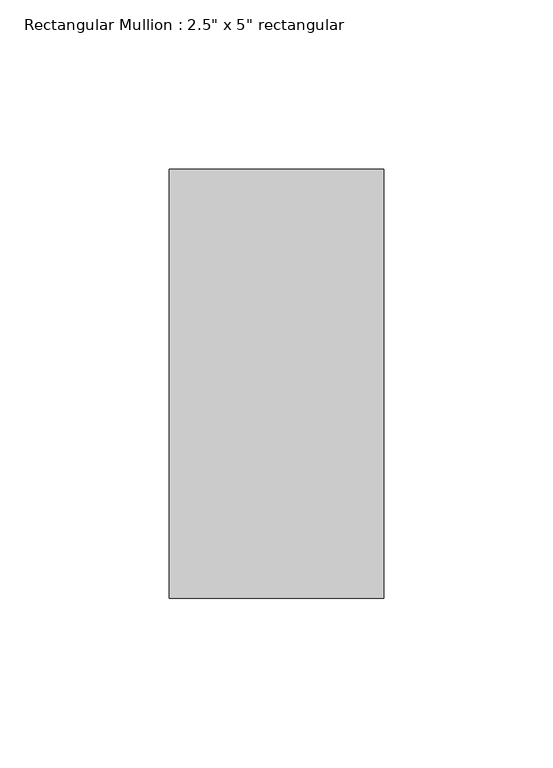
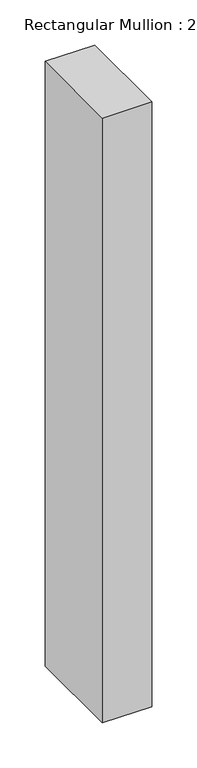
"""IFC4 building model written with IfcOpenShell, lengths in millimetres: member geometry."""

from ifc_helpers import new_model, si_unit, frame, origin, place, context, project, spatial, polyline, outline, extrude, source, transform, mapped, element, save


def member_3e1d4a65(model_context):
    return source(origin(), model_context, "Body", "SweptSolid", [
        extrude(outline(polyline([(0.0, 63.5), (0.0, -63.5), (-63.5, -63.5), (-63.5, 63.5), (0.0, 63.5)])), frame((0.0, 0.0, -819.5522598), z_axis=(0.0, 0.0, 1.0), x_axis=(1.0, 0.0, 0.0)), (0.0, 0.0, 1.0), 819.5522598),
    ])


if __name__ == "__main__":
    model = new_model("IFC4")
    model_context = context("Model", 3, world=origin())
    ifc_project = project(units=[si_unit("LENGTHUNIT", "METRE", prefix="MILLI")], contexts=[model_context])
    site = spatial("IfcSite", under=ifc_project)
    building = spatial("IfcBuilding", under=site)
    placement = place(None, origin())
    member_shape = member_3e1d4a65(model_context)
    element("IfcMember", 1, ObjectType="Rectangular Mullion : 2.5\" x 5\" rectangular", at=placement, inside=building, context=model_context, shape_type="MappedRepresentation", body=[
        mapped(member_shape, transform((0.0, 0.0, 0.0), x_axis=(1.0, 0.0, 0.0), y_axis=(0.0, 1.0, 0.0), z_axis=(0.0, 0.0, 1.0))),
    ])
    save(model, "model.ifc")

# Revit data of these elements
# Type "Rectangular Mullion : 2.5\" x 5\" rectangular"
#   built-in parameter 1007304 = 0.416667 (stored number, unit not read)
#   built-in parameter 1007301 = 0.104167 (stored number, unit not read)
#   built-in parameter 1007300 = 0.104167 (stored number, unit not read)
# Element 1 (IfcMember, "Rectangular Mullion : 2.5\" x 5\" rectangular")
#   Materials on its faces: "Aluminum"
# Materials
#   "Aluminum": class "Metal", colour RGB 247 247 247, transparency 0, Description = "Aluminum 6061", Cost = 0
